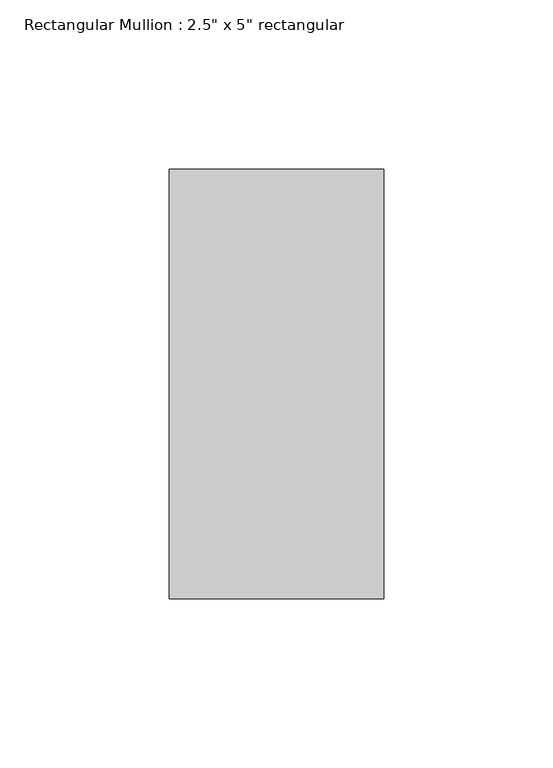
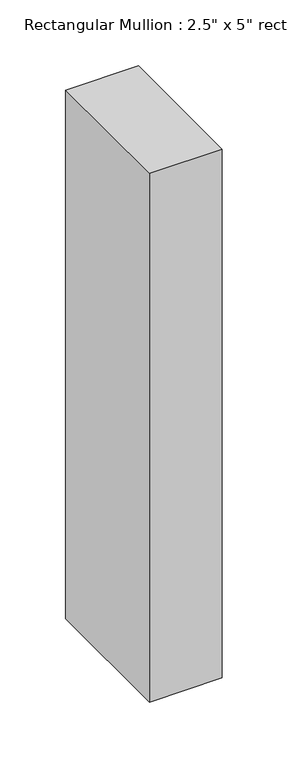
"""IFC4 building model written with IfcOpenShell, lengths in millimetres: member geometry."""

from ifc_helpers import new_model, si_unit, frame, origin, place, context, project, spatial, polyline, outline, extrude, source, transform, mapped, element, save


def member_b9f3750b(model_context):
    return source(origin(), model_context, "Body", "SweptSolid", [
        extrude(outline(polyline([(0.0, 63.5), (0.0, -63.5), (-63.5, -63.5), (-63.5, 63.5), (0.0, 63.5)])), frame((0.0, 0.0, -488.95), z_axis=(0.0, 0.0, 1.0), x_axis=(1.0, 0.0, 0.0)), (0.0, 0.0, 1.0), 488.95),
    ])


if __name__ == "__main__":
    model = new_model("IFC4")
    model_context = context("Model", 3, world=origin())
    ifc_project = project(units=[si_unit("LENGTHUNIT", "METRE", prefix="MILLI")], contexts=[model_context])
    site = spatial("IfcSite", under=ifc_project)
    building = spatial("IfcBuilding", under=site)
    placement = place(None, origin())
    member_shape = member_b9f3750b(model_context)
    element("IfcMember", 1, ObjectType="Rectangular Mullion : 2.5\" x 5\" rectangular", at=placement, inside=building, context=model_context, shape_type="MappedRepresentation", body=[
        mapped(member_shape, transform((0.0, 0.0, 0.0), x_axis=(1.0, 0.0, 0.0), y_axis=(0.0, 1.0, 0.0), z_axis=(0.0, 0.0, 1.0))),
    ])
    save(model, "model.ifc")

# Revit data of these elements
# Type "Rectangular Mullion : 2.5\" x 5\" rectangular"
#   built-in parameter 1007304 = 0.416667 (stored number, unit not read)
#   built-in parameter 1007301 = 0.104167 (stored number, unit not read)
#   built-in parameter 1007300 = 0.104167 (stored number, unit not read)
# Element 1 (IfcMember, "Rectangular Mullion : 2.5\" x 5\" rectangular")
#   Materials on its faces: "Aluminum"
# Materials
#   "Aluminum": class "Metal", colour RGB 247 247 247, transparency 0, Description = "Aluminum 6061", Cost = 0
